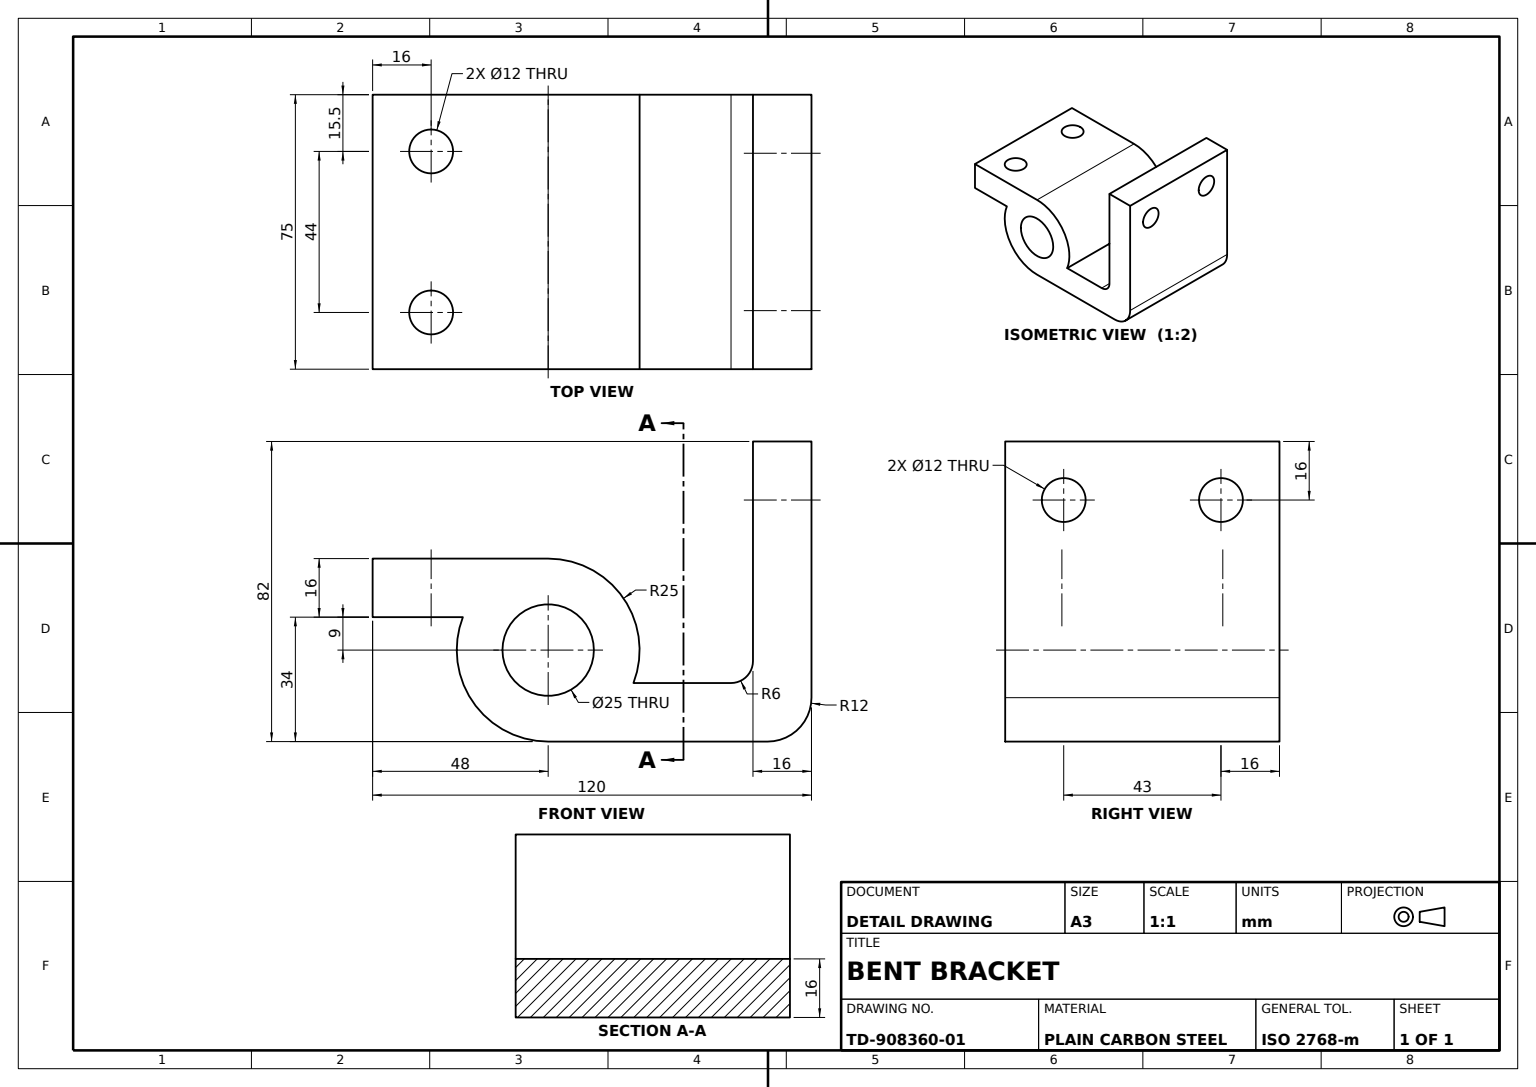
from build123d import *

# Parameters (mm, degrees)
BRACKET_BODY_DEPTH      = 75
FLANGE_A_HOLES_SKETCH_R = 6
FLANGE_A_HOLES_2X_DEPTH = 75
FLANGE_B_HOLES_SKETCH_R = 6
FLANGE_B_HOLES_2X_DEPTH = 75
PIVOT_BORE_SKETCH_R     = 12.5
PIVOT_BORE_DEPTH        = 75


with BuildPart() as part:
    # Bracket Profile Sketch → Bracket Body (new body)
    with BuildSketch(Plane.XY):
        with BuildLine():
            Line((0, -25), (60, -25))
            ThreePointArc((60, -25), (68.485281374, -21.485281374), (72, -13))
            Line((72, -13), (72, 57))
            Line((72, 57), (56, 57))
            Line((56, 57), (56, -3))
            ThreePointArc((56, -3), (54.242640687, -7.242640687), (50, -9))
            Line((50, -9), (23.323807579, -9))
            ThreePointArc((23.323807579, -9), (20.615528128, 14.142135624), (0, 25))
            Line((0, 25), (-48, 25))
            Line((-48, 25), (-48, 9))
            Line((-48, 9), (-23.323807579, 9))
            ThreePointArc((-23.323807579, 9), (-20.615528128, -14.142135624), (0, -25))
        make_face()
    extrude(amount=BRACKET_BODY_DEPTH)

    # Flange A Holes Sketch → Flange A Holes 2x (cut)
    with BuildSketch(Plane(origin=(0, 25, 0), x_dir=(1, 0, 0), z_dir=(0, 1, 0))):
        with Locations(Location((-32, -15.5, 0), (0, 0, 270))):
            Circle(FLANGE_A_HOLES_SKETCH_R)
        with Locations(Location((-32, -59.5, 0), (0, 0, 270))):
            Circle(FLANGE_A_HOLES_SKETCH_R)
    extrude(amount=-FLANGE_A_HOLES_2X_DEPTH, mode=Mode.SUBTRACT)

    # Flange B Holes Sketch → Flange B Holes 2x (cut)
    with BuildSketch(Plane(origin=(72, 0, 0), x_dir=(0, 0, -1), z_dir=(1, 0, 0))):
        with Locations((-59, 41)):
            Circle(FLANGE_B_HOLES_SKETCH_R)
        with Locations((-16, 41)):
            Circle(FLANGE_B_HOLES_SKETCH_R)
    extrude(amount=-FLANGE_B_HOLES_2X_DEPTH, mode=Mode.SUBTRACT)

    # Pivot Bore Sketch → Pivot Bore (cut)
    with BuildSketch(Plane.XY.offset(75)):
        Circle(PIVOT_BORE_SKETCH_R)
    extrude(amount=-PIVOT_BORE_DEPTH, mode=Mode.SUBTRACT)


solid = part.part
